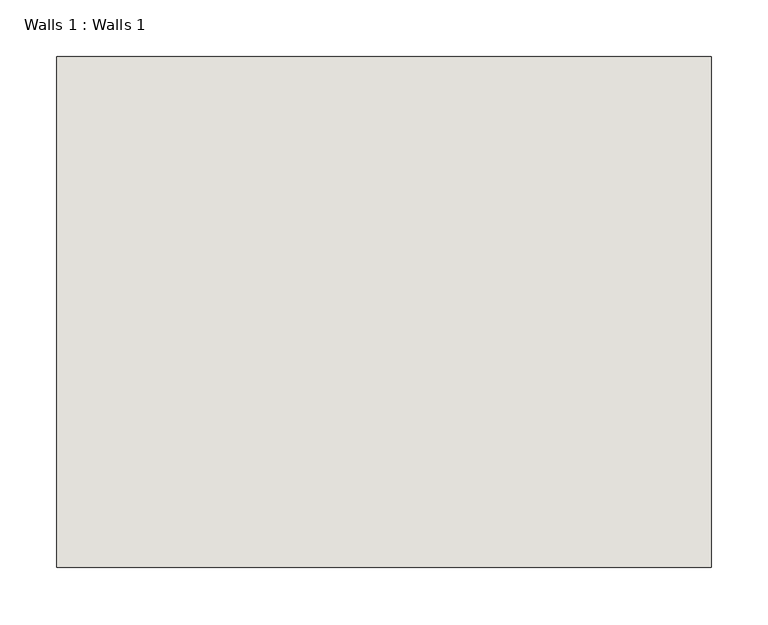
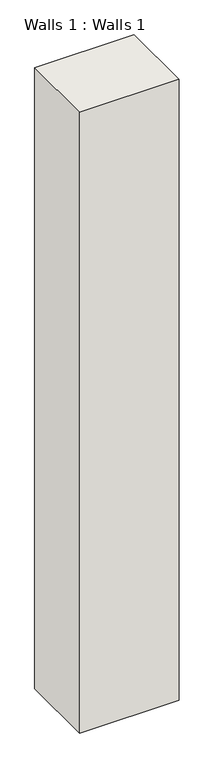
"""IFC4 building model written with IfcOpenShell, lengths in millimetres: wall geometry, Walls 1 : Walls 1."""

from ifc_helpers import new_model, si_unit, frame, origin, place, context, project, spatial, polyline, outline, extrude, source, transform, mapped, element, save


def walls_1_walls_1_84b2d317(model_context):
    return source(origin(), model_context, "Body", "SweptSolid", [
        extrude(outline(polyline([(-6654.9149176, 942.6953049), (-6077.6207252, 942.6953049), (-6077.6207252, 491.9864793), (-6654.9149176, 491.9864793), (-6654.9149176, 942.6953049)])), frame((0.0, 0.0, -1066.8), z_axis=(0.0, 0.0, 1.0), x_axis=(1.0, 0.0, 0.0)), (0.0, 0.0, 1.0), 3810.0),
    ])


if __name__ == "__main__":
    model = new_model("IFC4")
    model_context = context("Model", 3, world=origin())
    ifc_project = project(units=[si_unit("LENGTHUNIT", "METRE", prefix="MILLI")], contexts=[model_context])
    site = spatial("IfcSite", under=ifc_project)
    building = spatial("IfcBuilding", under=site)
    placement = place(None, origin())
    walls_1_walls_1_shape = walls_1_walls_1_84b2d317(model_context)
    element("IfcWall", 1, ObjectType="Walls 1 : Walls 1", at=placement, inside=building, context=model_context, shape_type="MappedRepresentation", body=[
        mapped(walls_1_walls_1_shape, transform((0.0, 0.0, 0.0), x_axis=(1.0, 0.0, 0.0), y_axis=(0.0, 1.0, 0.0), z_axis=(0.0, 0.0, 1.0))),
    ])
    save(model, "model.ifc")

# Revit data of these elements
# Element 1 (IfcWall, "Walls 1 : Walls 1")
#   Materials on its faces: "1 white", "Default Wall"
# Materials
#   "1 white": class "Generic", colour RGB 244 245 241, transparency 0, Cost = 0
#   "Default Wall": colour RGB 128 128 128, transparency 0, Cost = 0
